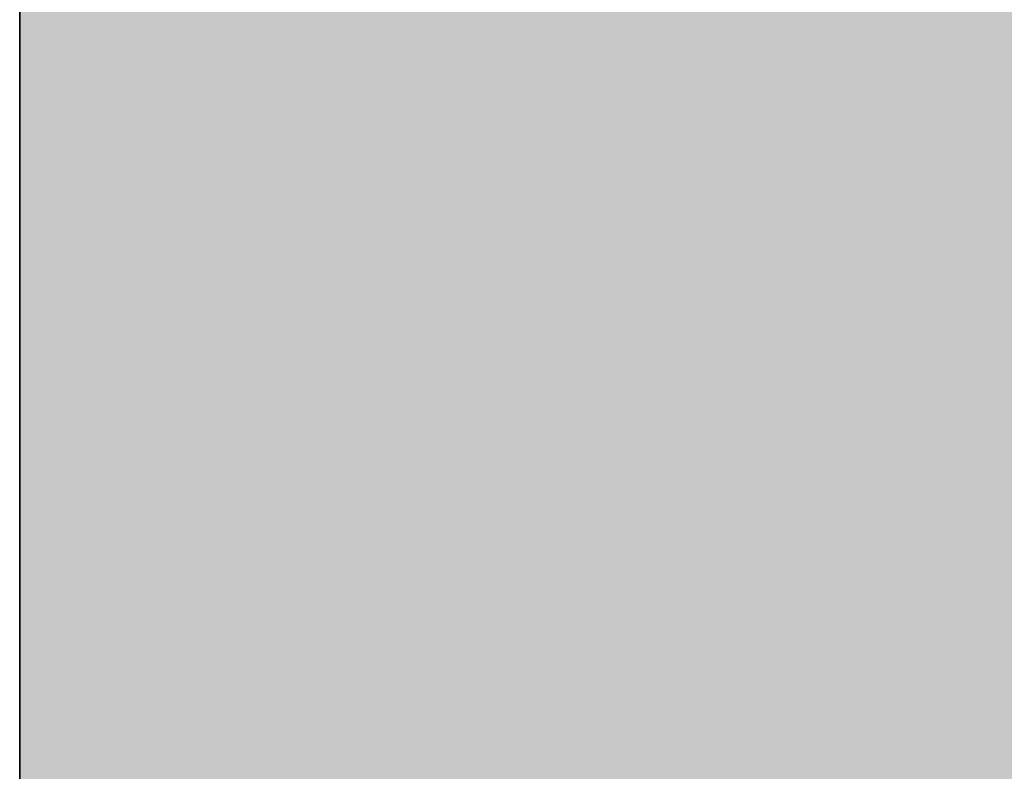
# Model space of a CAD drawing. Units: inches. Extents: x 2091 to 2899, y 967 to 2217.
# Tile 180 of 256: x 2203.1436 to 2203.16122, y 1152.26051 to 1152.27396. Entities that reach past the tile are written whole.
import ezdxf

# ---------------------------------------------------------------- set-up
doc = ezdxf.new("R2010")
doc.units = ezdxf.units.IN
doc.layers.add('A-WALL-PATT', color=141, linetype='Continuous', lineweight=13, true_color=0xadddf7)
doc.layers.add('C-PROP', color=7, linetype='Continuous', lineweight=35)

msp = doc.modelspace()

# ---------------------------------------------------------------- hatches: boundary and pattern name
at = {"layer": 'A-WALL-PATT'}
h = msp.add_hatch(color=256, dxfattribs=at)
h.dxf.hatch_style = 1
h.paths.add_polyline_path([(2803.143603, 2050.919059), (2203.143603, 2050.919059), (2203.143603, 1090.919059), (2803.143603, 1090.919059)])
h.paths.add_polyline_path([(2635.79885, 1147.540465), (2674.524052, 1147.540465, 0.376086), (2678.529665, 1152.880202), (2678.529665, 1159.556473, 0.333335), (2674.524319, 1163.561846), (2674.524319, 1163.56185), (2674.524319, 1192.93439), (2635.805971, 1192.93439), (2597.087622, 1192.93439), (2597.087622, 1163.561846, 0.333335), (2593.082276, 1159.556473), (2593.082276, 1152.880202, 0.376086), (2597.087889, 1147.540465)], flags=0)
h.paths.add_polyline_path([(2436.010433, 1278.240778, 0.000483), (2435.952643, 1278.215027, -0.001328), (2435.935625, 1278.111693, -0.001711), (2436.11644, 1278.040758, 0.002185)], flags=0)
h.paths.add_polyline_path([(2794.143603, 1143.419059), (2794.143603, 1347.419059), (2543.370171, 1347.419059), (2543.370171, 1351.919059), (2794.143603, 1351.919059), (2794.143603, 1392.713555), (2793.947398, 1392.713555), (2793.947398, 1473.5369), (2794.143603, 1473.5369), (2794.143603, 1531.919059), (2650.143603, 1531.919059), (2650.143603, 1536.419059), (2794.143603, 1536.419059), (2794.143603, 1692.419059), (2609.375609, 1692.419059), (2609.375609, 1644.419059), (2604.875609, 1644.419059), (2604.875609, 1744.919059), (2609.375609, 1744.919059), (2609.375609, 1696.919059), (2794.143603, 1696.919059), (2794.143603, 1780.919059), (2609.643603, 1780.919059), (2493.875609, 1780.919059), (2493.875609, 1785.419059), (2609.643603, 1785.419059), (2794.143603, 1785.419059), (2794.143603, 1847.938821), (2793.951222, 1847.938821), (2793.951222, 1928.762166), (2794.143603, 1928.762166), (2794.143603, 1941.419059), (2614.143603, 1941.419059), (2614.143603, 1821.419059), (2609.643603, 1821.419059), (2609.643603, 1941.419059), (2392.143603, 1941.419059), (2392.143603, 1819.919059), (2387.643603, 1819.919059), (2387.643603, 1941.419059), (2212.143603, 1941.419059), (2212.143603, 1783.919059), (2392.143603, 1783.919059), (2392.143603, 1780.919059), (2212.143603, 1780.919059), (2212.143603, 1629.419059), (2387.643603, 1629.419059), (2387.643603, 1744.919059), (2392.143603, 1744.919059), (2392.143603, 1627.919059), (2317.143603, 1627.919059), (2317.143603, 1551.419059), (2317.143603, 1536.419059), (2459.383591, 1536.419059), (2459.383591, 1602.39648), (2463.883591, 1602.39648), (2463.883591, 1531.919059), (2456.643603, 1531.919059), (2456.643603, 1529.919059), (2452.143603, 1529.919059), (2452.143603, 1531.919059), (2312.643603, 1531.919059), (2312.643603, 1551.419059), (2306.143603, 1551.419059), (2306.143603, 1555.919059), (2308.143603, 1555.919059), (2308.143603, 1551.419059), (2312.643603, 1551.419059), (2312.643603, 1627.919059), (2212.143603, 1627.919059), (2212.143603, 1555.919059), (2270.143603, 1555.919059), (2270.143603, 1551.419059), (2212.143603, 1551.419059), (2212.143603, 1351.919059), (2272.143603, 1351.919059), (2272.143603, 1347.419059), (2212.143603, 1347.419059), (2212.143603, 1275.419059), (2308.143603, 1275.419059), (2308.143603, 1351.919059), (2452.143603, 1351.919059), (2452.143603, 1493.919059), (2456.643603, 1493.919059), (2456.643603, 1347.419059), (2312.643603, 1347.419059), (2312.643603, 1270.919059), (2212.143603, 1270.919059), (2212.143603, 1099.919059), (2281.237523, 1099.919059), (2282.871041, 1110.913803), (2282.008341, 1116.996603), (2278.557741, 1121.420403), (2268.205641, 1128.056203), (2272.087641, 1128.056203), (2273.812941, 1131.927003), (2279.420341, 1134.691903), (2285.027841, 1135.244903), (2287.615841, 1137.456803), (2288.047141, 1138.009803), (2289.341141, 1140.774703), (2291.066541, 1139.668703), (2292.360541, 1135.244903), (2295.379841, 1136.903803), (2296.242541, 1135.797903), (2297.105241, 1133.033003), (2300.124641, 1138.009803), (2303.143941, 1138.009803), (2304.437941, 1135.797903), (2303.143941, 1133.586003), (2306.594641, 1134.691903), (2307.888741, 1133.033003), (2310.908041, 1135.244903), (2313.927441, 1134.138903), (2315.62686, 1132.427102), (2308.320041, 1117.549603), (2290.203841, 1109.807903), (2288.909841, 1103.172103), (2289.272309, 1099.919059), (2434.918227, 1099.919059), (2431.593227, 1124.788059), (2429.930227, 1169.553059), (2430.927185, 1240.519694), (2435.658926, 1238.186126), (2437.135227, 1196.554059), (2438.798227, 1143.973059), (2442.678227, 1111.998059), (2446.558227, 1099.919059), (2794.143603, 1099.919059), (2794.143603, 1138.919059), (2548.032447, 1138.919059), (2548.032447, 1143.419059), (2548.032447, 1148.819059), (2546.668457, 1148.031559), (2528.685692, 1179.178622, 0.256256), (2512.032447, 1148.819059), (2512.032447, 1143.419059), (2512.032447, 1138.919059), (2507.532447, 1138.919059), (2507.532447, 1143.419059), (2507.532447, 1148.819059, 0.256256), (2490.879202, 1179.178622), (2472.896437, 1148.031559), (2471.532447, 1148.819059), (2471.532447, 1143.419059), (2467.032447, 1143.419059), (2467.032447, 1269.945786, 0.039061), (2460.909987, 1273.580059), (2467.032447, 1273.580059), (2467.032447, 1286.325364, 0.014511), (2465.216194, 1286.761905), (2467.032447, 1287.052576), (2467.032447, 1323.419059), (2471.532447, 1323.419059), (2471.532447, 1148.819059), (2489.532447, 1179.995973), (2490.896437, 1179.208473), (2490.879202, 1179.178622, -0.256256), (2507.532447, 1148.819059), (2507.532447, 1143.419059), (2512.032447, 1143.419059), (2512.032447, 1148.819059, -0.256256), (2528.685692, 1179.178622), (2528.668457, 1179.208473), (2530.032447, 1179.995973), (2548.032447, 1148.819059), (2548.032447, 1143.419059)], flags=16)
h.paths.add_polyline_path([(2607.768546, 1200.945083), (2607.768546, 1265.030625), (2597.087622, 1281.052011), (2619.784585, 1281.052011), (2627.795278, 1337.12686), (2635.79885, 1337.12686), (2643.816663, 1337.12686), (2651.827356, 1281.052011), (2674.524319, 1281.052011), (2663.843395, 1265.030625), (2663.843395, 1200.945083), (2635.805971, 1200.945083)], flags=0)
edge = h.paths.add_edge_path(flags=0)
edge.add_ellipse((13303.896215, 1272.998725), major_axis=(-10595.31304, 0.000001), ratio=0.842303870086, start_angle=0.6282372191, end_angle=0.6465540999, ccw=False)
edge.add_ellipse((2711.70045, 1156.852678), major_axis=(2.219769, 0), ratio=0.84230387, start_angle=111.535244, end_angle=180.628237, ccw=False)
edge.add_ellipse((13303.156292, 1272.998725), major_axis=(-10593.026306, 0), ratio=0.842303869544, start_angle=0.5282714718, end_angle=0.6465540971, ccw=False)
edge.add_line((2710.764596, 1175.333295), (2710.129986, 1175.333295))
edge.add_ellipse((2710.129986, 1176.579775), major_axis=(1.479846, 0), ratio=0.84230387, start_angle=180, end_angle=270, ccw=False)
edge.add_line((2708.65014, 1176.579775), (2708.65014, 1200.782914))
edge.add_ellipse((2710.129986, 1200.782914), major_axis=(1.479846, 0), ratio=0.84230387, start_angle=90, end_angle=180, ccw=False)
edge.add_line((2710.129986, 1202.029394), (2710.465075, 1202.029394))
edge.add_ellipse((13303.156292, 1272.998725), major_axis=(-10593.026306, 0), ratio=0.842303869544, start_angle=-0.0902290886, end_angle=0.3838667788, ccw=False)
edge.add_ellipse((2710.129986, 1290.927031), major_axis=(-1.479846, 0), ratio=0.84230387, start_angle=0, end_angle=90, ccw=False)
edge.add_line((2708.65014, 1290.927031), (2708.65014, 1315.13017))
edge.add_ellipse((2710.129986, 1315.13017), major_axis=(-1.479846, 0), ratio=0.84230387, start_angle=-90, end_angle=0, ccw=False)
edge.add_line((2710.129986, 1316.37665), (2710.706314, 1316.37665))
edge.add_ellipse((3238.40172, 1296.289566), major_axis=(528.234, 0), ratio=0.8423038695, start_angle=176.34957241, end_angle=177.82004969, ccw=False)
edge.add_ellipse((2775.063043, 1071.450696), major_axis=(313.307761, 0), ratio=0.8423038695, start_angle=102.12596555, end_angle=103.78052899, ccw=False)
edge.add_ellipse((2775.063043, 1078.305698), major_axis=(-305.302891, 0), ratio=0.8423038695, start_angle=-79.790461, end_angle=-77.55537271, ccw=False)
edge.add_ellipse((2695.141767, 1541.975383), major_axis=(-250.960216, 0), ratio=0.8423038695, start_angle=99.25656601, end_angle=102.55493264)
edge.add_line((2741.410326, 1334.214255), (2747.132545, 1337.378477))
edge.add_ellipse((2747.538616, 1336.857478), major_axis=(-0.739923, 0), ratio=0.8423039, start_angle=270, end_angle=307.93313, ccw=False)
edge.add_ellipse((2747.538616, 1336.857478), major_axis=(-0.739923, 0), ratio=0.8423039, start_angle=232.06687, end_angle=270, ccw=False)
edge.add_line((2747.944687, 1337.378477), (2753.666906, 1334.214255))
edge.add_ellipse((2799.935466, 1541.975383), major_axis=(250.960216, 0), ratio=0.8423038695, start_angle=257.44506736, end_angle=260.74343399)
edge.add_ellipse((2720.014189, 1078.305698), major_axis=(305.302891, 0), ratio=0.8423038695, start_angle=77.55537271, end_angle=79.790461, ccw=False)
edge.add_ellipse((2720.014189, 1071.450696), major_axis=(-313.307761, 0), ratio=0.8423038695, start_angle=256.21947101, end_angle=257.87403445, ccw=False)
edge.add_ellipse((2256.675512, 1296.289566), major_axis=(-528.234, 0), ratio=0.8423038695, start_angle=182.17995031, end_angle=183.65042759, ccw=False)
edge.add_line((2784.370918, 1316.37665), (2784.947247, 1316.37665))
edge.add_ellipse((2784.947247, 1315.13017), major_axis=(1.479846, 0), ratio=0.84230387, start_angle=0, end_angle=90, ccw=False)
edge.add_line((2786.427093, 1315.13017), (2786.427093, 1290.927031))
edge.add_ellipse((2784.947247, 1290.927031), major_axis=(1.479846, 0), ratio=0.84230387, start_angle=270, end_angle=360, ccw=False)
edge.add_ellipse((-7808.07906, 1272.998725), major_axis=(10593.026306, 0), ratio=0.842303869544, start_angle=-0.3838667788, end_angle=0.0902290886, ccw=False)
edge.add_line((2784.612157, 1202.029394), (2784.947247, 1202.029394))
edge.add_ellipse((2784.947247, 1200.782914), major_axis=(1.479846, 0), ratio=0.84230387, start_angle=0, end_angle=90, ccw=False)
edge.add_line((2786.427093, 1200.782914), (2786.427093, 1176.579775))
edge.add_ellipse((2784.947247, 1176.579775), major_axis=(-1.479846, 0), ratio=0.84230387, start_angle=90, end_angle=180, ccw=False)
edge.add_line((2784.947247, 1175.333295), (2784.312636, 1175.333295))
edge.add_ellipse((-7808.07906, 1272.998725), major_axis=(10593.026306, 0), ratio=0.842303869544, start_angle=-0.6186431963, end_angle=-0.5282714718, ccw=False)
edge.add_ellipse((2783.376783, 1156.852678), major_axis=(-2.219769, 0), ratio=0.84230387, start_angle=179.371763, end_angle=248.464757, ccw=False)
edge.add_ellipse((-7808.818983, 1272.998725), major_axis=(-10595.31304, 0.000004), ratio=0.842303865762, start_angle=179.3534459226, end_angle=179.3717628034, ccw=False)
edge.add_ellipse((2780.297303, 1153.500793), major_axis=(-5.246426, 0), ratio=0.84230387, start_angle=90, end_angle=179.353446, ccw=False)
edge.add_line((2780.297303, 1149.081708), (2714.77993, 1149.081708))
edge.add_ellipse((2714.77993, 1153.500793), major_axis=(5.246426, 0), ratio=0.84230387, start_angle=180.646554, end_angle=270, ccw=False)
edge = h.paths.add_edge_path(flags=0)
edge.add_line((2718.187367, 1151.007833), (2718.187367, 1170.472364))
edge.add_ellipse((2721.14706, 1170.472364), major_axis=(-2.959692, 0), ratio=0.84230387, start_angle=-90, end_angle=0, ccw=False)
edge.add_line((2721.14706, 1172.965324), (2773.930173, 1172.965324))
edge.add_ellipse((2773.930173, 1170.472364), major_axis=(-2.959692, 0), ratio=0.84230387, start_angle=180, end_angle=270, ccw=False)
edge.add_line((2776.889865, 1170.472364), (2776.889865, 1151.007833))
edge.add_line((2776.889865, 1151.007833), (2718.187367, 1151.007833))
edge = h.paths.add_edge_path(flags=0)
edge.add_line((2718.187367, 1180.23415), (2718.187367, 1199.057834))
edge.add_ellipse((2747.538616, 1320.39864), major_axis=(147.017924, 0), ratio=0.8423038695, start_angle=256.40186531, end_angle=283.59813469)
edge.add_line((2776.889865, 1199.057834), (2776.889865, 1180.23415))
edge.add_ellipse((2747.538616, 1301.574956), major_axis=(147.017924, 0), ratio=0.8423038695, start_angle=256.40186531, end_angle=283.59813469, ccw=False)
edge = h.paths.add_edge_path(flags=0)
edge.add_ellipse((13303.156292, 1272.998725), major_axis=(-10591.54646, 0), ratio=0.842303869555, start_angle=0.0555943135, end_angle=0.3777641939, ccw=False)
edge.add_line((2711.616859, 1262.72171), (2715.667408, 1249.495396))
edge.add_ellipse((6413.891963, 1241.691919), major_axis=(-3698.236159, 0), ratio=0.84230386955, start_angle=-0.120897369, end_angle=0.364076349)
edge.add_line((2715.761038, 1218.192455), (2711.934307, 1203.167361))
edge = h.paths.add_edge_path(flags=0)
edge.add_line((2718.187367, 1251.074566), (2716.002485, 1267.450435))
edge.add_ellipse((2742.151175, 1202.18954), major_axis=(81.772585, 0), ratio=0.84230387, start_angle=94.27742096, end_angle=111.8349538, ccw=False)
edge.add_line((2737.009748, 1270.930626), (2758.067484, 1270.930626))
edge.add_ellipse((2752.926058, 1202.18954), major_axis=(81.772585, 0), ratio=0.84230387, start_angle=68.1650462, end_angle=85.72257904, ccw=False)
edge.add_line((2779.074747, 1267.450435), (2776.889865, 1251.074566))
edge.add_ellipse((2750.338059, 1187.885356), major_axis=(79.579664, 0), ratio=0.84230387, start_angle=67.20808512, end_angle=85.1299304)
edge.add_line((2756.034656, 1254.743656), (2739.042576, 1254.743656))
edge.add_ellipse((2744.739174, 1187.885356), major_axis=(79.579664, 0), ratio=0.84230387, start_angle=94.8700696, end_angle=112.79191488)
edge = h.paths.add_edge_path(flags=0)
edge.add_line((2783.142926, 1203.167361), (2779.316194, 1218.192455))
edge.add_ellipse((-918.81473, 1241.691919), major_axis=(3698.236159, 0), ratio=0.84230386955, start_angle=-0.364076349, end_angle=0.120897369)
edge.add_line((2779.409825, 1249.495396), (2783.460373, 1262.72171))
edge.add_ellipse((-7808.07906, 1272.998725), major_axis=(-10591.54646, 0), ratio=0.84230386954, start_angle=179.6222358061, end_angle=179.9444056865, ccw=False)
edge = h.paths.add_edge_path(flags=0)
edge.add_ellipse((2734.200892, 1286.69044), major_axis=(-0.356609, 6.340078), ratio=0.60383358, start_angle=89.0020143, end_angle=253.657408, ccw=False)
edge.add_line((2730.369001, 1286.541806), (2730.369001, 1301.35198))
edge.add_line((2730.369001, 1301.35198), (2735.913311, 1305.214803))
edge.add_ellipse((2736.384917, 1304.734561), major_axis=(0.739923, 0), ratio=0.8423039, start_angle=90, end_angle=134.480211, ccw=False)
edge.add_line((2736.384917, 1305.357801), (2738.032783, 1305.357801))
edge.add_line((2738.032783, 1305.357801), (2738.032783, 1307.707927))
edge.add_ellipse((2794.201642, 1307.707927), major_axis=(56.168859, 0), ratio=0.84230387, start_angle=150.5614304, end_angle=180, ccw=False)
edge.add_ellipse((2700.875591, 1307.707927), major_axis=(-56.168859, 0), ratio=0.84230387, start_angle=180, end_angle=209.4385696, ccw=False)
edge.add_line((2757.04445, 1307.707927), (2757.04445, 1305.357801))
edge.add_line((2757.04445, 1305.357801), (2758.692316, 1305.357801))
edge.add_ellipse((2758.692316, 1304.734561), major_axis=(-0.739923, 0), ratio=0.8423039, start_angle=225.519789, end_angle=270, ccw=False)
edge.add_line((2759.163922, 1305.214803), (2764.708231, 1301.35198))
edge.add_line((2764.708231, 1301.35198), (2764.708231, 1286.541806))
edge.add_ellipse((2760.87634, 1286.69044), major_axis=(0.356609, 6.340078), ratio=0.60383358, start_angle=106.342592, end_angle=270.9979857, ccw=False)
edge.add_line((2757.04445, 1285.79709), (2757.04445, 1307.707927))
edge.add_ellipse((2700.875591, 1307.707927), major_axis=(-56.168859, 0), ratio=0.84230387, start_angle=180, end_angle=209.4385696)
edge.add_ellipse((2794.201642, 1307.707927), major_axis=(56.168859, 0), ratio=0.84230387, start_angle=150.5614304, end_angle=180)
edge.add_line((2738.032783, 1307.707927), (2738.032783, 1285.79709))
h.paths.add_polyline_path([(2417.812273, 1104.449704), (2413.492273, 1102.529704), (2410.612273, 1103.969704), (2409.172273, 1106.369704), (2407.252273, 1107.329704), (2406.292273, 1109.729704), (2405.332273, 1114.049704), (2405.332273, 1117.889704), (2406.292273, 1120.129704), (2407.252273, 1119.809704), (2408.848322, 1118.327658), (2410.173945, 1119.42417), (2410.211273, 1120.405704), (2411.040731, 1121.419054), (2410.699273, 1119.858704), (2410.173945, 1119.42417), (2410.088452, 1117.176109), (2411.132836, 1116.206324), (2413.972273, 1119.329704), (2416.852273, 1120.769704), (2416.869721, 1120.798784), (2417.035071, 1119.405116), (2417.896213, 1118.143384), (2418.292273, 1118.369704), (2419.544447, 1120.039269), (2419.360915, 1118.387487), (2419.032108, 1119.356151), (2418.398939, 1118.511926), (2419.252273, 1114.529704), (2418.794091, 1107.198795)], flags=0)
h.paths.add_polyline_path([(2508.870171, 1347.419059), (2508.370171, 1347.419059), (2508.370171, 1351.919059), (2508.870171, 1351.919059)], flags=0)
h.paths.add_polyline_path([(2473.370171, 1347.419059), (2472.370171, 1347.419059), (2467.870171, 1347.419059), (2467.870171, 1455.419059), (2472.370171, 1455.419059), (2472.370171, 1352.419059), (2473.370171, 1352.419059)], flags=0)
h.paths.add_polyline_path([(2352.106244, 1217.446197), (2349.226244, 1218.886197), (2347.786244, 1221.286197), (2345.866244, 1222.246197), (2344.906244, 1224.646197), (2343.946244, 1228.966197), (2343.946244, 1232.806197), (2344.906244, 1235.046197), (2345.866244, 1234.726197), (2347.462293, 1233.244152), (2348.787916, 1234.340663), (2348.825244, 1235.322197), (2349.654702, 1236.335547), (2349.313244, 1234.775197), (2348.787916, 1234.340663), (2348.702423, 1232.092603), (2349.746807, 1231.122817), (2352.586244, 1234.246197), (2355.466244, 1235.686197), (2355.483692, 1235.715277), (2355.649043, 1234.321609), (2356.510185, 1233.059877), (2356.906244, 1233.286197), (2358.158418, 1234.955762), (2357.974887, 1233.30398), (2357.646079, 1234.272644), (2357.012911, 1233.428419), (2357.866244, 1229.446197), (2357.408062, 1222.115288), (2356.426244, 1219.366197)], flags=0)
h.paths.add_polyline_path([(2348.2968, 1112.22442), (2347.0138, 1112.31042), (2345.5298, 1114.12742), (2345.7318, 1115.85842), (2346.8118, 1116.98242), (2346.8118, 1114.64642), (2345.8668, 1114.21442), (2346.8798, 1114.30042)], flags=0)
h.paths.add_polyline_path([(2347.0138, 1110.92642), (2346.2718, 1110.49342), (2346.6098, 1111.18642)], flags=0)
h.paths.add_polyline_path([(2345.8668, 1118.19442), (2345.5298, 1117.32942), (2343.7078, 1118.02142), (2344.3828, 1118.62642)], flags=0)
h.paths.add_polyline_path([(2346.6768, 1109.28242), (2346.0698, 1108.07142), (2345.8668, 1110.06142)], flags=0)
h.paths.add_polyline_path([(2345.0568, 1119.75142), (2343.6398, 1119.75142), (2343.9778, 1121.13542)], flags=0)
h.paths.add_polyline_path([(2345.2598, 1116.55042), (2345.1248, 1115.85842), (2344.9218, 1115.68542), (2344.7198, 1116.37742)], flags=0)
h.paths.add_polyline_path([(2345.6648, 1112.31042), (2345.4618, 1111.53242), (2344.0448, 1111.96442), (2344.6518, 1112.57042)], flags=0)
h.paths.add_polyline_path([(2345.1918, 1113.34942), (2344.4498, 1113.86842), (2344.7198, 1114.38742)], flags=0)
h.paths.add_polyline_path([(2344.6518, 1116.80942), (2344.1798, 1115.68542), (2344.6518, 1115.33942), (2343.9098, 1114.90642), (2343.0328, 1115.94442), (2343.6398, 1116.46342)], flags=0)
h.paths.add_polyline_path([(2345.8668, 1106.68642), (2344.9898, 1105.56242), (2344.5168, 1106.60042)], flags=0)
h.paths.add_polyline_path([(2344.8548, 1110.06142), (2344.5168, 1109.28242), (2344.1128, 1109.71542)], flags=0)
h.paths.add_polyline_path([(2344.0448, 1113.52242), (2343.4378, 1113.08942), (2342.7628, 1113.95442)], flags=0)
h.paths.add_polyline_path([(2344.3148, 1111.01242), (2342.9648, 1110.32042), (2342.9648, 1111.09942)], flags=0)
h.paths.add_polyline_path([(2345.1248, 1104.69742), (2344.5848, 1103.74542), (2344.4498, 1104.26442)], flags=0)
h.paths.add_polyline_path([(2342.8298, 1121.22242), (2341.7498, 1120.53042), (2340.5358, 1121.04942), (2340.1308, 1121.82842), (2340.6708, 1122.95242), (2341.1428, 1121.82842), (2341.6148, 1122.00142)], flags=0)
h.paths.add_polyline_path([(2342.9648, 1119.75142), (2343.0328, 1118.45342), (2342.0878, 1118.02142), (2342.0198, 1119.49142)], flags=0)
h.paths.add_polyline_path([(2342.6948, 1116.89642), (2341.9528, 1116.63642), (2342.0198, 1117.32942)], flags=0)
h.paths.add_polyline_path([(2343.0328, 1112.22442), (2342.0198, 1111.79142), (2341.5478, 1112.22442), (2342.3578, 1113.34942)], flags=0)
h.paths.add_polyline_path([(2343.7748, 1104.43742), (2342.6278, 1102.88042), (2342.6948, 1104.61042), (2343.4378, 1105.12942)], flags=0)
h.paths.add_polyline_path([(2342.0198, 1115.07942), (2340.8058, 1115.51242), (2340.9408, 1116.37742)], flags=0)
h.paths.add_polyline_path([(2341.4808, 1120.09742), (2341.4808, 1119.40542), (2341.0758, 1119.57842), (2341.1428, 1120.09742)], flags=0)
h.paths.add_polyline_path([(2341.8178, 1114.47342), (2340.9408, 1113.08942), (2340.8058, 1114.56042)], flags=0)
h.paths.add_polyline_path([(2341.1428, 1118.54042), (2340.9408, 1116.98242), (2339.0508, 1117.67542), (2339.0508, 1118.62642)], flags=0)
h.paths.add_polyline_path([(2342.6948, 1101.66842), (2341.9528, 1101.84142), (2342.5598, 1102.36142)], flags=0)
h.paths.add_polyline_path([(2340.3328, 1119.66542), (2338.4438, 1119.57842), (2337.9038, 1120.35742), (2339.6578, 1120.61642)], flags=0)
h.paths.add_polyline_path([(2340.3328, 1115.33942), (2340.0628, 1113.69542), (2339.3878, 1115.33942)], flags=0)
h.paths.add_polyline_path([(2341.8178, 1103.83142), (2341.5478, 1102.88042), (2341.1428, 1103.65842)], flags=0)
h.paths.add_polyline_path([(2339.0508, 1122.86642), (2337.2958, 1121.82842), (2337.0938, 1123.12542), (2337.7688, 1123.81842)], flags=0)
h.paths.add_polyline_path([(2339.1178, 1121.74142), (2338.8478, 1121.22242), (2338.1738, 1121.04942), (2338.3758, 1121.56842)], flags=0)
h.paths.add_polyline_path([(2339.1858, 1119.31942), (2338.6458, 1118.71342), (2338.2408, 1118.10742), (2338.2408, 1118.88642)], flags=0)
h.paths.add_polyline_path([(2341.1428, 1101.92842), (2340.6028, 1101.23642), (2340.0628, 1101.84142), (2340.6028, 1102.36142)], flags=0)
h.paths.add_polyline_path([(2337.6338, 1117.76142), (2336.6208, 1118.28042), (2337.2958, 1118.97242)], flags=0)
h.paths.add_polyline_path([(2336.8238, 1119.57842), (2334.7988, 1118.97242), (2335.2038, 1120.35742), (2336.5538, 1120.87642)], flags=0)
h.paths.add_polyline_path([(2339.1178, 1100.45742), (2337.3638, 1100.54342), (2336.7558, 1101.23642)], flags=0)
h.paths.add_polyline_path([(2336.3508, 1122.43342), (2336.0138, 1121.91442), (2334.9338, 1122.43342), (2334.5288, 1123.47142), (2335.7438, 1122.77942)], flags=0)
h.paths.add_polyline_path([(2334.7318, 1120.87642), (2334.2588, 1120.35742), (2334.0568, 1120.78942), (2334.5968, 1121.30842)], flags=0)
h.paths.add_polyline_path([(2334.4618, 1122.17442), (2332.5718, 1121.30842), (2331.3568, 1122.17442), (2332.0998, 1122.86642)], flags=0)
h.paths.add_polyline_path([(2334.2588, 1118.54042), (2333.3818, 1118.45342), (2333.6518, 1119.31942)], flags=0)
h.paths.add_polyline_path([(2335.5418, 1102.27442), (2334.1918, 1102.62042), (2335.2718, 1103.31242)], flags=0)
h.paths.add_polyline_path([(2332.7068, 1119.66542), (2331.6948, 1120.44342), (2332.5048, 1120.78942)], flags=0)
h.paths.add_polyline_path([(2334.7318, 1101.14942), (2333.5168, 1101.58242), (2333.9888, 1101.75542)], flags=0)
h.paths.add_polyline_path([(2332.6398, 1116.63642), (2331.0868, 1116.29042), (2331.9648, 1118.19442)], flags=0)
h.paths.add_polyline_path([(2330.7498, 1121.56842), (2330.2768, 1120.27042), (2328.5228, 1119.31942), (2328.9948, 1121.04942)], flags=0)
h.paths.add_polyline_path([(2330.7498, 1118.62642), (2330.0078, 1117.50242), (2329.8728, 1118.02142)], flags=0)
h.paths.add_polyline_path([(2332.0998, 1102.36142), (2330.5468, 1102.01442), (2331.6948, 1102.96642)], flags=0)
h.paths.add_polyline_path([(2329.5348, 1113.60842), (2329.0628, 1112.31042), (2328.5898, 1113.34942)], flags=0)
h.paths.add_polyline_path([(2328.3878, 1117.84842), (2327.5098, 1116.55042), (2327.1728, 1117.76142)], flags=0)
h.paths.add_polyline_path([(2329.7378, 1106.51342), (2329.5348, 1105.30242), (2328.2528, 1106.08142)], flags=0)
h.paths.add_polyline_path([(2328.6578, 1114.38742), (2328.0498, 1114.12742), (2328.3198, 1114.90642)], flags=0)
h.paths.add_polyline_path([(2328.3198, 1112.22442), (2327.1058, 1112.13742), (2326.7008, 1112.65642)], flags=0)
h.paths.add_polyline_path([(2326.9028, 1115.25242), (2326.7008, 1114.12742), (2325.2158, 1113.60842), (2326.0928, 1115.33942)], flags=0)
h.paths.add_polyline_path([(2326.6328, 1108.33042), (2326.0928, 1107.37942), (2325.8908, 1108.50342), (2326.4978, 1109.10942)], flags=0)
h.paths.add_polyline_path([(2615.143603, 1531.919059), (2609.643603, 1531.919059), (2609.643603, 1620.419059), (2614.143603, 1620.419059), (2614.143603, 1536.419059), (2615.143603, 1536.419059)], flags=0)
h.paths.add_polyline_path([(2545.143603, 1563.419059), (2464.143603, 1563.419059), (2464.143603, 1632.419059), (2509.143603, 1632.419059), (2509.143603, 1627.919059), (2509.143603, 1603.919059), (2468.643603, 1603.919059), (2468.643603, 1567.919059), (2540.643603, 1567.919059), (2540.643603, 1591.919059), (2545.143603, 1591.919059)], flags=0)
h.paths.add_polyline_path([(2388.969048, 1549.985735), (2357.434181, 1549.985735), (2357.434181, 1623.360778), (2399.362777, 1623.360778), (2435.689465, 1623.360778), (2435.592547, 1602.559273), (2435.592547, 1602.39648), (2388.969048, 1602.39648)], flags=0)
h.paths.add_polyline_path([(2388.880628, 1555.809151), (2374.904429, 1555.809151), (2374.904429, 1600.571564), (2374.904429, 1615.457645), (2406.350877, 1615.457645), (2406.350877, 1618.939431), (2412.174293, 1615.457645), (2406.350877, 1611.97586), (2406.350877, 1615.457645), (2388.880628, 1615.457645)], flags=0)
h.paths.add_polyline_path([(2568.875609, 1644.419059), (2453.375609, 1644.419059), (2453.375609, 1785.419059), (2457.875609, 1785.419059), (2457.875609, 1648.919059), (2568.875609, 1648.919059)], flags=0)
h.paths.add_polyline_path([(2212.143603, 1945.919059), (2212.143603, 2041.919059), (2794.143603, 2041.919059), (2794.143603, 1945.919059)], flags=16)
h.paths.add_polyline_path([(2271.082728, 1964.317238), (2776.852968, 1964.317238), (2776.852968, 2037.169623), (2271.082728, 2037.169623)], flags=8)
h.paths.add_polyline_path([(2380.649285, 1536.824144), (2461.040809, 1536.824144), (2461.040809, 1554.652587), (2380.649285, 1554.652587)], flags=8)
h.paths.add_polyline_path([(2240.755709, 1609.725451), (2309.185829, 1609.725451), (2309.185829, 1617.698204), (2240.755709, 1617.698204)], flags=8)
h.paths.add_polyline_path([(2212.677255, 1313.504102), (2282.59152, 1313.504102), (2282.59152, 1322.745239), (2212.677255, 1322.745239)], flags=8)
h.paths.add_polyline_path([(2457.111976, 1114.778574), (2558.481581, 1114.778574), (2558.481581, 1142.219682), (2457.111976, 1142.219682)], flags=8)
h.paths.add_polyline_path([(2473.442337, 1273.010067), (2604.641226, 1273.010067), (2604.641226, 1318.346935), (2473.442337, 1318.346935)], flags=8)
h.paths.add_polyline_path([(2638.876302, 1626.977432), (2684.250367, 1627.976738), (2684.038483, 1637.597494), (2638.664417, 1636.598188)], flags=8)
h.paths.add_polyline_path([(2537.590554, 1453.793447), (2628.389547, 1453.793447), (2628.389547, 1475.344811), (2537.590554, 1475.344811)], flags=8)
h.paths.add_polyline_path([(2504.137638, 1714.632397), (2554.647187, 1714.632397), (2554.647187, 1730.237712), (2504.137638, 1730.237712)], flags=8)
h.paths.add_polyline_path([(2487.501181, 1575.651872), (2535.097121, 1575.651872), (2535.097121, 1598.377646), (2487.501181, 1598.377646)], flags=8)
h.paths.add_polyline_path([(2709.0994, 1735.710278), (2740.016601, 1735.710278), (2740.016601, 1749.937641), (2709.0994, 1749.937641)], flags=8)
h.paths.add_polyline_path([(2442.438424, 1792.171657), (2564.728835, 1792.171657), (2564.728835, 1842.000163), (2442.438424, 1842.000163)], flags=8)
h.paths.add_polyline_path([(2655.815801, 1809.644076), (2789.520142, 1806.693796), (2790.084977, 1832.291638), (2656.380635, 1835.241918)], flags=8)
h.paths.add_polyline_path([(2234.842697, 1797.720143), (2368.592851, 1794.768852), (2369.160718, 1820.504132), (2235.410564, 1823.455423)], flags=8)
h.paths.add_polyline_path([(2245.138466, 1644.006335), (2398.427733, 1640.6239), (2398.994842, 1666.32482), (2245.705575, 1669.707255)], flags=8)
h.paths.add_polyline_path([(2306.142847, 1431.168519), (2413.768314, 1428.793687), (2414.333148, 1454.391529), (2306.707682, 1456.76636)], flags=8)
h.paths.add_polyline_path([(2306.834582, 1458.233145), (2393.380484, 1456.323449), (2393.932808, 1481.354358), (2307.386907, 1483.264054)], flags=8)

# ---------------------------------------------------------------- linework, layer by layer
at = {"layer": 'C-PROP'}
msp.add_lwpolyline([(2203.143603, 2050.919059), (2803.143603, 2050.919059), (2803.143603, 1090.919059), (2203.143603, 1090.919059)], close=True, dxfattribs=at)

doc.saveas('drawing.dxf')
